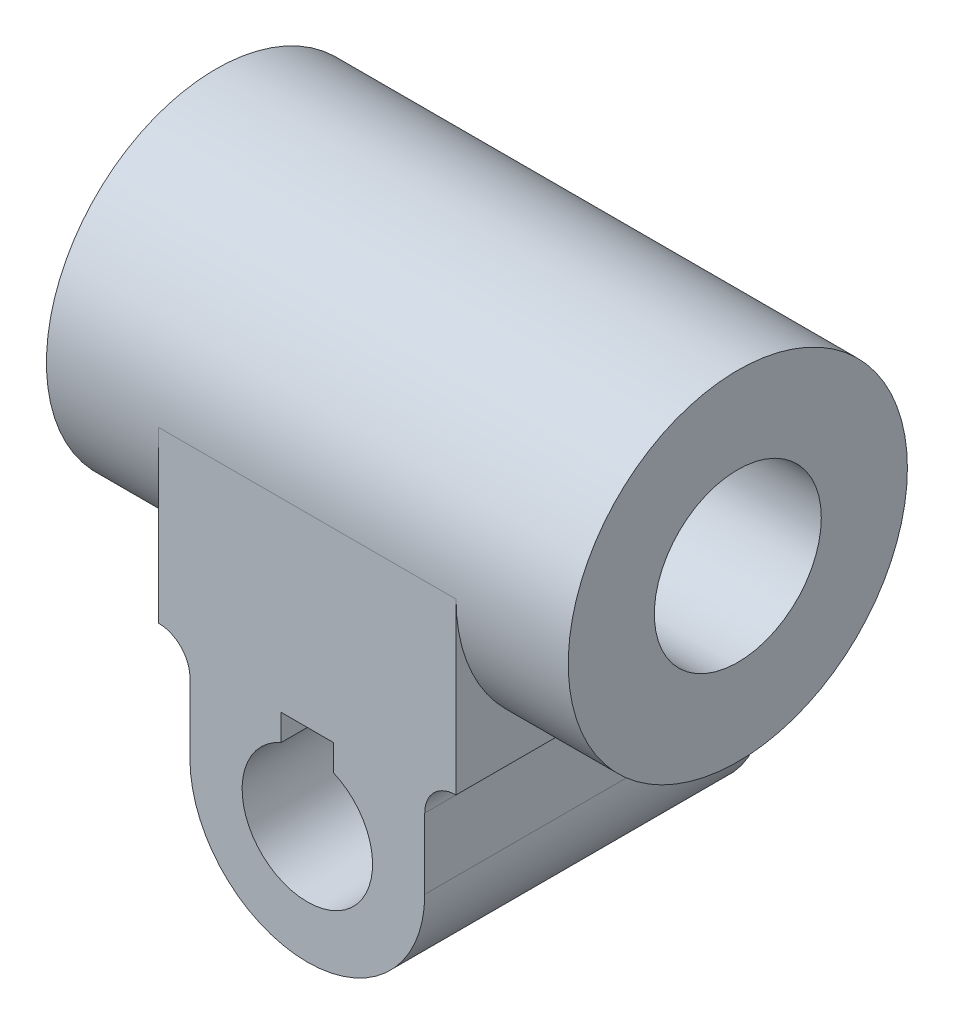
ISO-10303-21;
HEADER;
FILE_DESCRIPTION(('STEP AP214'),'2;1');
FILE_NAME('part.step','',(''),(''),'','','');
FILE_SCHEMA(('AUTOMOTIVE_DESIGN { 1 0 10303 214 1 1 1 1 }'));
ENDSEC;
DATA;
#1=APPLICATION_CONTEXT('core data for automotive mechanical design processes');
#2=APPLICATION_PROTOCOL_DEFINITION('international standard','automotive_design',2000,#1);
#3=PRODUCT_CONTEXT('',#1,'mechanical');
#4=PRODUCT('Part','Part','',(#3));
#5=PRODUCT_RELATED_PRODUCT_CATEGORY('part','',(#4));
#6=PRODUCT_DEFINITION_FORMATION('','',#4);
#7=PRODUCT_DEFINITION_CONTEXT('part definition',#1,'design');
#8=PRODUCT_DEFINITION('design','',#6,#7);
#9=PRODUCT_DEFINITION_SHAPE('','',#8);
#10=(LENGTH_UNIT() NAMED_UNIT(*) SI_UNIT(.MILLI.,.METRE.));
#11=(NAMED_UNIT(*) PLANE_ANGLE_UNIT() SI_UNIT($,.RADIAN.));
#12=(NAMED_UNIT(*) SI_UNIT($,.STERADIAN.) SOLID_ANGLE_UNIT());
#13=UNCERTAINTY_MEASURE_WITH_UNIT(LENGTH_MEASURE(1.E-05),#10,'distance_accuracy_value','');
#14=(GEOMETRIC_REPRESENTATION_CONTEXT(3) GLOBAL_UNCERTAINTY_ASSIGNED_CONTEXT((#13)) GLOBAL_UNIT_ASSIGNED_CONTEXT((#10,
#11,#12)) REPRESENTATION_CONTEXT('',''));
#15=CARTESIAN_POINT('',(0.,0.,0.));
#16=DIRECTION('',(0.,0.,1.));
#17=DIRECTION('',(1.,0.,0.));
#18=AXIS2_PLACEMENT_3D('',#15,#16,#17);
#19=CARTESIAN_POINT('',(50.,0.,0.));
#20=DIRECTION('',(-1.,0.,0.));
#21=DIRECTION('',(0.,0.,1.));
#22=AXIS2_PLACEMENT_3D('',#19,#20,#21);
#23=CYLINDRICAL_SURFACE('',#22,32.5);
#24=CARTESIAN_POINT('',(-50.,0.,0.));
#25=DIRECTION('',(1.,0.,0.));
#26=DIRECTION('',(0.,0.,-1.));
#27=AXIS2_PLACEMENT_3D('',#24,#25,#26);
#28=CIRCLE('',#27,32.5);
#29=CARTESIAN_POINT('',(-50.,0.,-32.5));
#30=VERTEX_POINT('',#29);
#31=EDGE_CURVE('E42',#30,#30,#28,.T.);
#32=ORIENTED_EDGE('',*,*,#31,.T.);
#33=EDGE_LOOP('',(#32));
#34=FACE_BOUND('',#33,.T.);
#35=CARTESIAN_POINT('',(50.,0.,0.));
#36=DIRECTION('',(1.,0.,0.));
#37=DIRECTION('',(0.,0.,-1.));
#38=AXIS2_PLACEMENT_3D('',#35,#36,#37);
#39=CIRCLE('',#38,32.5);
#40=CARTESIAN_POINT('',(50.,0.,-32.5));
#41=VERTEX_POINT('',#40);
#42=EDGE_CURVE('E11',#41,#41,#39,.T.);
#43=ORIENTED_EDGE('',*,*,#42,.F.);
#44=EDGE_LOOP('',(#43));
#45=FACE_BOUND('',#44,.T.);
#46=CARTESIAN_POINT('',(-28.5,0.,0.));
#47=DIRECTION('',(1.,0.,0.));
#48=DIRECTION('',(0.,1.,0.));
#49=AXIS2_PLACEMENT_3D('',#46,#47,#48);
#50=CIRCLE('',#49,32.5);
#51=CARTESIAN_POINT('',(-28.5,0.,32.5));
#52=VERTEX_POINT('',#51);
#53=CARTESIAN_POINT('',(-28.5,-32.5,0.));
#54=VERTEX_POINT('',#53);
#55=EDGE_CURVE('E241',#52,#54,#50,.T.);
#56=ORIENTED_EDGE('',*,*,#55,.F.);
#57=DIRECTION('',(1.,0.,0.));
#58=VECTOR('',#57,1.);
#59=CARTESIAN_POINT('',(0.,0.,32.5));
#60=LINE('',#59,#58);
#61=CARTESIAN_POINT('',(28.5,0.,32.5));
#62=VERTEX_POINT('',#61);
#63=EDGE_CURVE('E208',#52,#62,#60,.T.);
#64=ORIENTED_EDGE('',*,*,#63,.T.);
#65=CARTESIAN_POINT('',(28.5,0.,0.));
#66=DIRECTION('',(1.,0.,0.));
#67=DIRECTION('',(0.,1.,0.));
#68=AXIS2_PLACEMENT_3D('',#65,#66,#67);
#69=CIRCLE('',#68,32.5);
#70=CARTESIAN_POINT('',(28.5,-32.5,0.));
#71=VERTEX_POINT('',#70);
#72=EDGE_CURVE('E244',#62,#71,#69,.T.);
#73=ORIENTED_EDGE('',*,*,#72,.T.);
#74=CARTESIAN_POINT('',(28.5,0.,-32.5));
#75=VERTEX_POINT('',#74);
#76=EDGE_CURVE('E224',#71,#75,#69,.T.);
#77=ORIENTED_EDGE('',*,*,#76,.T.);
#78=DIRECTION('',(1.,0.,0.));
#79=VECTOR('',#78,1.);
#80=CARTESIAN_POINT('',(0.,0.,-32.5));
#81=LINE('',#80,#79);
#82=CARTESIAN_POINT('',(-28.5,0.,-32.5));
#83=VERTEX_POINT('',#82);
#84=EDGE_CURVE('E58',#83,#75,#81,.T.);
#85=ORIENTED_EDGE('',*,*,#84,.F.);
#86=EDGE_CURVE('E54',#54,#83,#50,.T.);
#87=ORIENTED_EDGE('',*,*,#86,.F.);
#88=EDGE_LOOP('',(#56,#64,#73,#77,#85,#87));
#89=FACE_BOUND('',#88,.T.);
#90=ADVANCED_FACE('F41',(#34,#45,#89),#23,.T.);
#91=CARTESIAN_POINT('',(50.,0.,0.));
#92=DIRECTION('',(-1.,0.,0.));
#93=DIRECTION('',(0.,0.,1.));
#94=AXIS2_PLACEMENT_3D('',#91,#92,#93);
#95=CYLINDRICAL_SURFACE('',#94,16.);
#96=CARTESIAN_POINT('',(50.,0.,0.));
#97=DIRECTION('',(1.,0.,0.));
#98=DIRECTION('',(0.,0.,-1.));
#99=AXIS2_PLACEMENT_3D('',#96,#97,#98);
#100=CIRCLE('',#99,16.);
#101=CARTESIAN_POINT('',(50.,0.,-16.));
#102=VERTEX_POINT('',#101);
#103=EDGE_CURVE('E243',#102,#102,#100,.T.);
#104=ORIENTED_EDGE('',*,*,#103,.T.);
#105=EDGE_LOOP('',(#104));
#106=FACE_BOUND('',#105,.T.);
#107=CARTESIAN_POINT('',(-50.,0.,0.));
#108=DIRECTION('',(1.,0.,0.));
#109=DIRECTION('',(0.,0.,-1.));
#110=AXIS2_PLACEMENT_3D('',#107,#108,#109);
#111=CIRCLE('',#110,16.);
#112=CARTESIAN_POINT('',(-50.,0.,-16.));
#113=VERTEX_POINT('',#112);
#114=EDGE_CURVE('E248',#113,#113,#111,.T.);
#115=ORIENTED_EDGE('',*,*,#114,.F.);
#116=EDGE_LOOP('',(#115));
#117=FACE_BOUND('',#116,.T.);
#118=ADVANCED_FACE('F294',(#106,#117),#95,.F.);
#119=CARTESIAN_POINT('',(50.,0.,0.));
#120=DIRECTION('',(1.,0.,0.));
#121=DIRECTION('',(0.,0.,-1.));
#122=AXIS2_PLACEMENT_3D('',#119,#120,#121);
#123=PLANE('',#122);
#124=ORIENTED_EDGE('',*,*,#42,.T.);
#125=EDGE_LOOP('',(#124));
#126=FACE_BOUND('',#125,.T.);
#127=ORIENTED_EDGE('',*,*,#103,.F.);
#128=EDGE_LOOP('',(#127));
#129=FACE_BOUND('',#128,.T.);
#130=ADVANCED_FACE('F298',(#126,#129),#123,.T.);
#131=CARTESIAN_POINT('',(-50.,0.,0.));
#132=DIRECTION('',(1.,0.,0.));
#133=DIRECTION('',(0.,0.,-1.));
#134=AXIS2_PLACEMENT_3D('',#131,#132,#133);
#135=PLANE('',#134);
#136=ORIENTED_EDGE('',*,*,#31,.F.);
#137=EDGE_LOOP('',(#136));
#138=FACE_BOUND('',#137,.T.);
#139=ORIENTED_EDGE('',*,*,#114,.T.);
#140=EDGE_LOOP('',(#139));
#141=FACE_BOUND('',#140,.T.);
#142=ADVANCED_FACE('F287',(#138,#141),#135,.F.);
#143=CARTESIAN_POINT('',(-28.5,0.,-32.5));
#144=DIRECTION('',(1.,0.,0.));
#145=DIRECTION('',(0.,1.,0.));
#146=AXIS2_PLACEMENT_3D('',#143,#144,#145);
#147=PLANE('',#146);
#148=DIRECTION('',(0.,1.,0.));
#149=VECTOR('',#148,1.);
#150=CARTESIAN_POINT('',(-28.5,0.,32.5));
#151=LINE('',#150,#149);
#152=CARTESIAN_POINT('',(-28.5,-32.5,32.5));
#153=VERTEX_POINT('',#152);
#154=EDGE_CURVE('E209',#153,#52,#151,.T.);
#155=ORIENTED_EDGE('',*,*,#154,.T.);
#156=ORIENTED_EDGE('',*,*,#55,.T.);
#157=DIRECTION('',(0.,0.,1.));
#158=VECTOR('',#157,1.);
#159=CARTESIAN_POINT('',(-28.5,-32.5,-32.5));
#160=LINE('',#159,#158);
#161=EDGE_CURVE('E231',#54,#153,#160,.T.);
#162=ORIENTED_EDGE('',*,*,#161,.T.);
#163=EDGE_LOOP('',(#155,#156,#162));
#164=FACE_BOUND('',#163,.T.);
#165=ADVANCED_FACE('F251',(#164),#147,.F.);
#166=CARTESIAN_POINT('',(28.5,0.,-32.5));
#167=DIRECTION('',(1.,0.,0.));
#168=DIRECTION('',(0.,1.,0.));
#169=AXIS2_PLACEMENT_3D('',#166,#167,#168);
#170=PLANE('',#169);
#171=ORIENTED_EDGE('',*,*,#72,.F.);
#172=DIRECTION('',(0.,1.,0.));
#173=VECTOR('',#172,1.);
#174=CARTESIAN_POINT('',(28.5,0.,32.5));
#175=LINE('',#174,#173);
#176=CARTESIAN_POINT('',(28.5,-32.5,32.5));
#177=VERTEX_POINT('',#176);
#178=EDGE_CURVE('E202',#177,#62,#175,.T.);
#179=ORIENTED_EDGE('',*,*,#178,.F.);
#180=DIRECTION('',(0.,0.,1.));
#181=VECTOR('',#180,1.);
#182=CARTESIAN_POINT('',(28.5,-32.5,-32.5));
#183=LINE('',#182,#181);
#184=EDGE_CURVE('E234',#71,#177,#183,.T.);
#185=ORIENTED_EDGE('',*,*,#184,.F.);
#186=EDGE_LOOP('',(#171,#179,#185));
#187=FACE_BOUND('',#186,.T.);
#188=ADVANCED_FACE('F279',(#187),#170,.T.);
#189=CARTESIAN_POINT('',(0.,-52.,-32.5));
#190=DIRECTION('',(0.,0.,1.));
#191=DIRECTION('',(1.,0.,0.));
#192=AXIS2_PLACEMENT_3D('',#189,#190,#191);
#193=CYLINDRICAL_SURFACE('',#192,12.5);
#194=CARTESIAN_POINT('',(0.,-52.,32.5));
#195=DIRECTION('',(0.,0.,1.));
#196=DIRECTION('',(1.,0.,0.));
#197=AXIS2_PLACEMENT_3D('',#194,#195,#196);
#198=CIRCLE('',#197,12.5);
#199=CARTESIAN_POINT('',(5.,-40.5435607626104,32.5));
#200=VERTEX_POINT('',#199);
#201=CARTESIAN_POINT('',(-4.99999999999998,-40.5435607626104,32.5));
#202=VERTEX_POINT('',#201);
#203=EDGE_CURVE('E213',#200,#202,#198,.F.);
#204=ORIENTED_EDGE('',*,*,#203,.F.);
#205=DIRECTION('',(0.,0.,1.));
#206=VECTOR('',#205,1.);
#207=CARTESIAN_POINT('',(5.,-40.5435607626104,-32.5));
#208=LINE('',#207,#206);
#209=CARTESIAN_POINT('',(5.,-40.5435607626104,-32.5));
#210=VERTEX_POINT('',#209);
#211=EDGE_CURVE('E222',#210,#200,#208,.T.);
#212=ORIENTED_EDGE('',*,*,#211,.F.);
#213=CARTESIAN_POINT('',(0.,-52.,-32.5));
#214=DIRECTION('',(0.,0.,1.));
#215=DIRECTION('',(1.,0.,0.));
#216=AXIS2_PLACEMENT_3D('',#213,#214,#215);
#217=CIRCLE('',#216,12.5);
#218=CARTESIAN_POINT('',(-4.99999999999998,-40.5435607626104,-32.5));
#219=VERTEX_POINT('',#218);
#220=EDGE_CURVE('E185',#210,#219,#217,.F.);
#221=ORIENTED_EDGE('',*,*,#220,.T.);
#222=DIRECTION('',(0.,0.,1.));
#223=VECTOR('',#222,1.);
#224=CARTESIAN_POINT('',(-4.99999999999998,-40.5435607626104,-32.5));
#225=LINE('',#224,#223);
#226=EDGE_CURVE('E230',#219,#202,#225,.T.);
#227=ORIENTED_EDGE('',*,*,#226,.T.);
#228=EDGE_LOOP('',(#204,#212,#221,#227));
#229=FACE_BOUND('',#228,.T.);
#230=ADVANCED_FACE('F278',(#229),#193,.F.);
#231=CARTESIAN_POINT('',(5.00000000000002,0.,-32.5));
#232=DIRECTION('',(-1.,0.,0.));
#233=DIRECTION('',(0.,-1.,0.));
#234=AXIS2_PLACEMENT_3D('',#231,#232,#233);
#235=PLANE('',#234);
#236=DIRECTION('',(0.,-1.,0.));
#237=VECTOR('',#236,1.);
#238=CARTESIAN_POINT('',(5.00000000000002,0.,32.5));
#239=LINE('',#238,#237);
#240=CARTESIAN_POINT('',(5.,-35.5435607626104,32.5));
#241=VERTEX_POINT('',#240);
#242=EDGE_CURVE('E162',#241,#200,#239,.T.);
#243=ORIENTED_EDGE('',*,*,#242,.F.);
#244=DIRECTION('',(0.,0.,1.));
#245=VECTOR('',#244,1.);
#246=CARTESIAN_POINT('',(5.,-35.5435607626104,-32.5));
#247=LINE('',#246,#245);
#248=CARTESIAN_POINT('',(5.,-35.5435607626104,-32.5));
#249=VERTEX_POINT('',#248);
#250=EDGE_CURVE('E221',#249,#241,#247,.T.);
#251=ORIENTED_EDGE('',*,*,#250,.F.);
#252=DIRECTION('',(0.,-1.,0.));
#253=VECTOR('',#252,1.);
#254=CARTESIAN_POINT('',(5.00000000000002,0.,-32.5));
#255=LINE('',#254,#253);
#256=EDGE_CURVE('E156',#249,#210,#255,.T.);
#257=ORIENTED_EDGE('',*,*,#256,.T.);
#258=ORIENTED_EDGE('',*,*,#211,.T.);
#259=EDGE_LOOP('',(#243,#251,#257,#258));
#260=FACE_BOUND('',#259,.T.);
#261=ADVANCED_FACE('F286',(#260),#235,.T.);
#262=CARTESIAN_POINT('',(0.,-35.5435607626104,-32.5));
#263=DIRECTION('',(0.,-1.,0.));
#264=DIRECTION('',(0.,0.,-1.));
#265=AXIS2_PLACEMENT_3D('',#262,#263,#264);
#266=PLANE('',#265);
#267=DIRECTION('',(1.,0.,0.));
#268=VECTOR('',#267,1.);
#269=CARTESIAN_POINT('',(0.,-35.5435607626104,32.5));
#270=LINE('',#269,#268);
#271=CARTESIAN_POINT('',(-5.,-35.5435607626104,32.5));
#272=VERTEX_POINT('',#271);
#273=EDGE_CURVE('E167',#272,#241,#270,.T.);
#274=ORIENTED_EDGE('',*,*,#273,.F.);
#275=DIRECTION('',(0.,0.,1.));
#276=VECTOR('',#275,1.);
#277=CARTESIAN_POINT('',(-5.,-35.5435607626104,-32.5));
#278=LINE('',#277,#276);
#279=CARTESIAN_POINT('',(-5.,-35.5435607626104,-32.5));
#280=VERTEX_POINT('',#279);
#281=EDGE_CURVE('E227',#280,#272,#278,.T.);
#282=ORIENTED_EDGE('',*,*,#281,.F.);
#283=DIRECTION('',(1.,0.,0.));
#284=VECTOR('',#283,1.);
#285=CARTESIAN_POINT('',(0.,-35.5435607626104,-32.5));
#286=LINE('',#285,#284);
#287=EDGE_CURVE('E190',#280,#249,#286,.T.);
#288=ORIENTED_EDGE('',*,*,#287,.T.);
#289=ORIENTED_EDGE('',*,*,#250,.T.);
#290=EDGE_LOOP('',(#274,#282,#288,#289));
#291=FACE_BOUND('',#290,.T.);
#292=ADVANCED_FACE('F317',(#291),#266,.T.);
#293=CARTESIAN_POINT('',(-28.5,-38.5,-32.5));
#294=DIRECTION('',(0.,0.,1.));
#295=DIRECTION('',(1.,0.,0.));
#296=AXIS2_PLACEMENT_3D('',#293,#294,#295);
#297=CYLINDRICAL_SURFACE('',#296,6.00000000000001);
#298=CARTESIAN_POINT('',(-28.5,-38.5,32.5));
#299=DIRECTION('',(0.,0.,1.));
#300=DIRECTION('',(1.,0.,0.));
#301=AXIS2_PLACEMENT_3D('',#298,#299,#300);
#302=CIRCLE('',#301,6.00000000000001);
#303=CARTESIAN_POINT('',(-22.5,-38.5,32.5));
#304=VERTEX_POINT('',#303);
#305=EDGE_CURVE('E193',#153,#304,#302,.F.);
#306=ORIENTED_EDGE('',*,*,#305,.F.);
#307=ORIENTED_EDGE('',*,*,#161,.F.);
#308=CARTESIAN_POINT('',(-28.5,-32.5,-32.5));
#309=VERTEX_POINT('',#308);
#310=EDGE_CURVE('E161',#309,#54,#160,.T.);
#311=ORIENTED_EDGE('',*,*,#310,.F.);
#312=CARTESIAN_POINT('',(-28.5,-38.5,-32.5));
#313=DIRECTION('',(0.,0.,1.));
#314=DIRECTION('',(1.,0.,0.));
#315=AXIS2_PLACEMENT_3D('',#312,#313,#314);
#316=CIRCLE('',#315,6.00000000000001);
#317=CARTESIAN_POINT('',(-22.5,-38.5,-32.5));
#318=VERTEX_POINT('',#317);
#319=EDGE_CURVE('E143',#309,#318,#316,.F.);
#320=ORIENTED_EDGE('',*,*,#319,.T.);
#321=DIRECTION('',(0.,0.,1.));
#322=VECTOR('',#321,1.);
#323=CARTESIAN_POINT('',(-22.5,-38.5,-32.5));
#324=LINE('',#323,#322);
#325=EDGE_CURVE('E146',#318,#304,#324,.T.);
#326=ORIENTED_EDGE('',*,*,#325,.T.);
#327=EDGE_LOOP('',(#306,#307,#311,#320,#326));
#328=FACE_BOUND('',#327,.T.);
#329=ADVANCED_FACE('F158',(#328),#297,.F.);
#330=ORIENTED_EDGE('',*,*,#310,.T.);
#331=ORIENTED_EDGE('',*,*,#86,.T.);
#332=DIRECTION('',(0.,1.,0.));
#333=VECTOR('',#332,1.);
#334=CARTESIAN_POINT('',(-28.5,0.,-32.5));
#335=LINE('',#334,#333);
#336=EDGE_CURVE('E179',#309,#83,#335,.T.);
#337=ORIENTED_EDGE('',*,*,#336,.F.);
#338=EDGE_LOOP('',(#330,#331,#337));
#339=FACE_BOUND('',#338,.T.);
#340=ADVANCED_FACE('F260',(#339),#147,.F.);
#341=ORIENTED_EDGE('',*,*,#76,.F.);
#342=CARTESIAN_POINT('',(28.5,-32.5,-32.5));
#343=VERTEX_POINT('',#342);
#344=EDGE_CURVE('E235',#343,#71,#183,.T.);
#345=ORIENTED_EDGE('',*,*,#344,.F.);
#346=DIRECTION('',(0.,1.,0.));
#347=VECTOR('',#346,1.);
#348=CARTESIAN_POINT('',(28.5,0.,-32.5));
#349=LINE('',#348,#347);
#350=EDGE_CURVE('E176',#343,#75,#349,.T.);
#351=ORIENTED_EDGE('',*,*,#350,.T.);
#352=EDGE_LOOP('',(#341,#345,#351));
#353=FACE_BOUND('',#352,.T.);
#354=ADVANCED_FACE('F261',(#353),#170,.T.);
#355=CARTESIAN_POINT('',(28.5,-38.5,-32.5));
#356=DIRECTION('',(0.,0.,1.));
#357=DIRECTION('',(1.,0.,0.));
#358=AXIS2_PLACEMENT_3D('',#355,#356,#357);
#359=CYLINDRICAL_SURFACE('',#358,6.00000000000001);
#360=CARTESIAN_POINT('',(28.5,-38.5,32.5));
#361=DIRECTION('',(0.,0.,1.));
#362=DIRECTION('',(1.,0.,0.));
#363=AXIS2_PLACEMENT_3D('',#360,#361,#362);
#364=CIRCLE('',#363,6.00000000000001);
#365=CARTESIAN_POINT('',(22.5,-38.5,32.5));
#366=VERTEX_POINT('',#365);
#367=EDGE_CURVE('E205',#366,#177,#364,.F.);
#368=ORIENTED_EDGE('',*,*,#367,.F.);
#369=DIRECTION('',(0.,0.,1.));
#370=VECTOR('',#369,1.);
#371=CARTESIAN_POINT('',(22.5,-38.5,-32.5));
#372=LINE('',#371,#370);
#373=CARTESIAN_POINT('',(22.5,-38.5,-32.5));
#374=VERTEX_POINT('',#373);
#375=EDGE_CURVE('E237',#374,#366,#372,.T.);
#376=ORIENTED_EDGE('',*,*,#375,.F.);
#377=CARTESIAN_POINT('',(28.5,-38.5,-32.5));
#378=DIRECTION('',(0.,0.,1.));
#379=DIRECTION('',(1.,0.,0.));
#380=AXIS2_PLACEMENT_3D('',#377,#378,#379);
#381=CIRCLE('',#380,6.00000000000001);
#382=EDGE_CURVE('E175',#374,#343,#381,.F.);
#383=ORIENTED_EDGE('',*,*,#382,.T.);
#384=ORIENTED_EDGE('',*,*,#344,.T.);
#385=ORIENTED_EDGE('',*,*,#184,.T.);
#386=EDGE_LOOP('',(#368,#376,#383,#384,#385));
#387=FACE_BOUND('',#386,.T.);
#388=ADVANCED_FACE('F264',(#387),#359,.F.);
#389=CARTESIAN_POINT('',(22.5,0.,-32.5));
#390=DIRECTION('',(1.,0.,0.));
#391=DIRECTION('',(0.,0.,-1.));
#392=AXIS2_PLACEMENT_3D('',#389,#390,#391);
#393=PLANE('',#392);
#394=DIRECTION('',(0.,1.,0.));
#395=VECTOR('',#394,1.);
#396=CARTESIAN_POINT('',(22.5,0.,32.5));
#397=LINE('',#396,#395);
#398=CARTESIAN_POINT('',(22.5,-52.,32.5));
#399=VERTEX_POINT('',#398);
#400=EDGE_CURVE('E200',#399,#366,#397,.T.);
#401=ORIENTED_EDGE('',*,*,#400,.F.);
#402=DIRECTION('',(0.,0.,1.));
#403=VECTOR('',#402,1.);
#404=CARTESIAN_POINT('',(22.5,-52.,-32.5));
#405=LINE('',#404,#403);
#406=CARTESIAN_POINT('',(22.5,-52.,-32.5));
#407=VERTEX_POINT('',#406);
#408=EDGE_CURVE('E236',#407,#399,#405,.T.);
#409=ORIENTED_EDGE('',*,*,#408,.F.);
#410=DIRECTION('',(0.,1.,0.));
#411=VECTOR('',#410,1.);
#412=CARTESIAN_POINT('',(22.5,0.,-32.5));
#413=LINE('',#412,#411);
#414=EDGE_CURVE('E168',#407,#374,#413,.T.);
#415=ORIENTED_EDGE('',*,*,#414,.T.);
#416=ORIENTED_EDGE('',*,*,#375,.T.);
#417=EDGE_LOOP('',(#401,#409,#415,#416));
#418=FACE_BOUND('',#417,.T.);
#419=ADVANCED_FACE('F267',(#418),#393,.T.);
#420=CARTESIAN_POINT('',(0.,-52.,-32.5));
#421=DIRECTION('',(0.,0.,1.));
#422=DIRECTION('',(1.,0.,0.));
#423=AXIS2_PLACEMENT_3D('',#420,#421,#422);
#424=CYLINDRICAL_SURFACE('',#423,22.5);
#425=CARTESIAN_POINT('',(0.,-52.,32.5));
#426=DIRECTION('',(0.,0.,1.));
#427=DIRECTION('',(1.,0.,0.));
#428=AXIS2_PLACEMENT_3D('',#425,#426,#427);
#429=CIRCLE('',#428,22.5);
#430=CARTESIAN_POINT('',(-22.5,-52.,32.5));
#431=VERTEX_POINT('',#430);
#432=EDGE_CURVE('E198',#431,#399,#429,.T.);
#433=ORIENTED_EDGE('',*,*,#432,.F.);
#434=DIRECTION('',(0.,0.,1.));
#435=VECTOR('',#434,1.);
#436=CARTESIAN_POINT('',(-22.5,-52.,-32.5));
#437=LINE('',#436,#435);
#438=CARTESIAN_POINT('',(-22.5,-52.,-32.5));
#439=VERTEX_POINT('',#438);
#440=EDGE_CURVE('E154',#439,#431,#437,.T.);
#441=ORIENTED_EDGE('',*,*,#440,.F.);
#442=CARTESIAN_POINT('',(0.,-52.,-32.5));
#443=DIRECTION('',(0.,0.,1.));
#444=DIRECTION('',(1.,0.,0.));
#445=AXIS2_PLACEMENT_3D('',#442,#443,#444);
#446=CIRCLE('',#445,22.5);
#447=EDGE_CURVE('E145',#439,#407,#446,.T.);
#448=ORIENTED_EDGE('',*,*,#447,.T.);
#449=ORIENTED_EDGE('',*,*,#408,.T.);
#450=EDGE_LOOP('',(#433,#441,#448,#449));
#451=FACE_BOUND('',#450,.T.);
#452=ADVANCED_FACE('F275',(#451),#424,.T.);
#453=CARTESIAN_POINT('',(-22.5,0.,-32.5));
#454=DIRECTION('',(1.,0.,0.));
#455=DIRECTION('',(0.,0.,-1.));
#456=AXIS2_PLACEMENT_3D('',#453,#454,#455);
#457=PLANE('',#456);
#458=DIRECTION('',(0.,1.,0.));
#459=VECTOR('',#458,1.);
#460=CARTESIAN_POINT('',(-22.5,0.,32.5));
#461=LINE('',#460,#459);
#462=EDGE_CURVE('E151',#431,#304,#461,.T.);
#463=ORIENTED_EDGE('',*,*,#462,.T.);
#464=ORIENTED_EDGE('',*,*,#325,.F.);
#465=DIRECTION('',(0.,1.,0.));
#466=VECTOR('',#465,1.);
#467=CARTESIAN_POINT('',(-22.5,0.,-32.5));
#468=LINE('',#467,#466);
#469=EDGE_CURVE('E131',#439,#318,#468,.T.);
#470=ORIENTED_EDGE('',*,*,#469,.F.);
#471=ORIENTED_EDGE('',*,*,#440,.T.);
#472=EDGE_LOOP('',(#463,#464,#470,#471));
#473=FACE_BOUND('',#472,.T.);
#474=ADVANCED_FACE('F149',(#473),#457,.F.);
#475=CARTESIAN_POINT('',(-5.00000000000001,0.,-32.5));
#476=DIRECTION('',(1.,0.,0.));
#477=DIRECTION('',(0.,1.,0.));
#478=AXIS2_PLACEMENT_3D('',#475,#476,#477);
#479=PLANE('',#478);
#480=DIRECTION('',(0.,1.,0.));
#481=VECTOR('',#480,1.);
#482=CARTESIAN_POINT('',(-5.00000000000001,0.,32.5));
#483=LINE('',#482,#481);
#484=EDGE_CURVE('E216',#202,#272,#483,.T.);
#485=ORIENTED_EDGE('',*,*,#484,.F.);
#486=ORIENTED_EDGE('',*,*,#226,.F.);
#487=DIRECTION('',(0.,1.,0.));
#488=VECTOR('',#487,1.);
#489=CARTESIAN_POINT('',(-5.00000000000001,0.,-32.5));
#490=LINE('',#489,#488);
#491=EDGE_CURVE('E183',#219,#280,#490,.T.);
#492=ORIENTED_EDGE('',*,*,#491,.T.);
#493=ORIENTED_EDGE('',*,*,#281,.T.);
#494=EDGE_LOOP('',(#485,#486,#492,#493));
#495=FACE_BOUND('',#494,.T.);
#496=ADVANCED_FACE('F325',(#495),#479,.T.);
#497=CARTESIAN_POINT('',(0.,0.,-32.5));
#498=DIRECTION('',(0.,0.,1.));
#499=DIRECTION('',(1.,0.,0.));
#500=AXIS2_PLACEMENT_3D('',#497,#498,#499);
#501=PLANE('',#500);
#502=ORIENTED_EDGE('',*,*,#350,.F.);
#503=ORIENTED_EDGE('',*,*,#382,.F.);
#504=ORIENTED_EDGE('',*,*,#414,.F.);
#505=ORIENTED_EDGE('',*,*,#447,.F.);
#506=ORIENTED_EDGE('',*,*,#469,.T.);
#507=ORIENTED_EDGE('',*,*,#319,.F.);
#508=ORIENTED_EDGE('',*,*,#336,.T.);
#509=ORIENTED_EDGE('',*,*,#84,.T.);
#510=EDGE_LOOP('',(#502,#503,#504,#505,#506,#507,#508,#509));
#511=FACE_BOUND('',#510,.T.);
#512=ORIENTED_EDGE('',*,*,#220,.F.);
#513=ORIENTED_EDGE('',*,*,#256,.F.);
#514=ORIENTED_EDGE('',*,*,#287,.F.);
#515=ORIENTED_EDGE('',*,*,#491,.F.);
#516=EDGE_LOOP('',(#512,#513,#514,#515));
#517=FACE_BOUND('',#516,.T.);
#518=ADVANCED_FACE('F140',(#511,#517),#501,.F.);
#519=CARTESIAN_POINT('',(0.,0.,32.5));
#520=DIRECTION('',(0.,0.,1.));
#521=DIRECTION('',(1.,0.,0.));
#522=AXIS2_PLACEMENT_3D('',#519,#520,#521);
#523=PLANE('',#522);
#524=ORIENTED_EDGE('',*,*,#154,.F.);
#525=ORIENTED_EDGE('',*,*,#305,.T.);
#526=ORIENTED_EDGE('',*,*,#462,.F.);
#527=ORIENTED_EDGE('',*,*,#432,.T.);
#528=ORIENTED_EDGE('',*,*,#400,.T.);
#529=ORIENTED_EDGE('',*,*,#367,.T.);
#530=ORIENTED_EDGE('',*,*,#178,.T.);
#531=ORIENTED_EDGE('',*,*,#63,.F.);
#532=EDGE_LOOP('',(#524,#525,#526,#527,#528,#529,#530,#531));
#533=FACE_BOUND('',#532,.T.);
#534=ORIENTED_EDGE('',*,*,#203,.T.);
#535=ORIENTED_EDGE('',*,*,#484,.T.);
#536=ORIENTED_EDGE('',*,*,#273,.T.);
#537=ORIENTED_EDGE('',*,*,#242,.T.);
#538=EDGE_LOOP('',(#534,#535,#536,#537));
#539=FACE_BOUND('',#538,.T.);
#540=ADVANCED_FACE('F273',(#533,#539),#523,.T.);
#541=CLOSED_SHELL('',(#90,#118,#130,#142,#165,#188,#230,#261,#292,#329,#340,#354,#388,#419,#452,
#474,#496,#518,#540));
#542=MANIFOLD_SOLID_BREP('B2',#541);
#543=ADVANCED_BREP_SHAPE_REPRESENTATION('',(#18,#542),#14);
#544=SHAPE_DEFINITION_REPRESENTATION(#9,#543);
ENDSEC;
END-ISO-10303-21;
